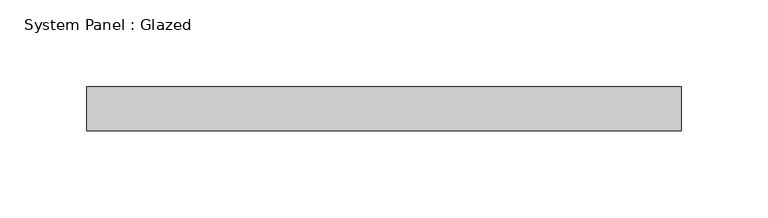
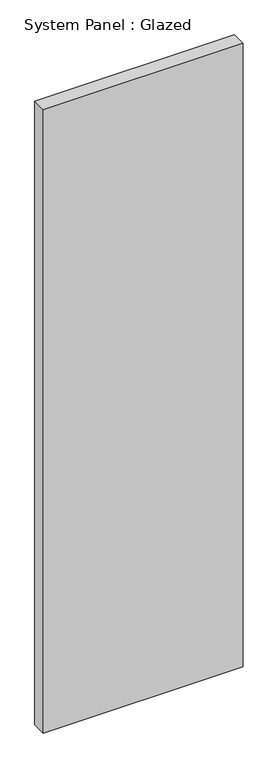
"""IFC4 building model written with IfcOpenShell, lengths in millimetres: plate geometry, System Panel : Glazed."""

from ifc_helpers import new_model, si_unit, origin, origin_with_axes, place, context, project, spatial, polyline, outline, extrude, source, transform, mapped, element, save


def system_panel_glazed_7089d882(model_context):
    return source(origin(), model_context, "Body", "SweptSolid", [
        extrude(outline(polyline([(171.45, 19.05), (-171.45, 19.05), (-171.45, 44.45), (171.45, 44.45), (171.45, 19.05)])), origin_with_axes(), (0.0, 0.0, 1.0), 1130.6019988),
    ])


if __name__ == "__main__":
    model = new_model("IFC4")
    model_context = context("Model", 3, world=origin())
    ifc_project = project(units=[si_unit("LENGTHUNIT", "METRE", prefix="MILLI")], contexts=[model_context])
    site = spatial("IfcSite", under=ifc_project)
    building = spatial("IfcBuilding", under=site)
    placement = place(None, origin())
    system_panel_glazed_shape = system_panel_glazed_7089d882(model_context)
    element("IfcPlate", 1, ObjectType="System Panel : Glazed", at=placement, inside=building, context=model_context, shape_type="MappedRepresentation", body=[
        mapped(system_panel_glazed_shape, transform((0.0, 0.0, 0.0), x_axis=(1.0, 0.0, 0.0), y_axis=(0.0, 1.0, 0.0), z_axis=(0.0, 0.0, 1.0))),
    ])
    save(model, "model.ifc")

# Revit data of these elements
# Type "System Panel : Glazed"
#   Construction Type Id = "GSP4R"
#   Analytic Construction = "1/8 in Pilkington single glazing"
#   Visual Light Transmittance = 0.9
#   Solar Heat Gain Coefficient = 0.86
#   Heat Transfer Coefficient (U) = 1.18115 BTU/(h·ft²·°F)
# Element 1 (IfcPlate, "System Panel : Glazed")
#   Materials on its faces: "Glass"
# Materials
#   "Glass": class "Glass", colour RGB 0 128 192, transparency 0.75, Description = "Soda Lime Glass", Cost = 0
